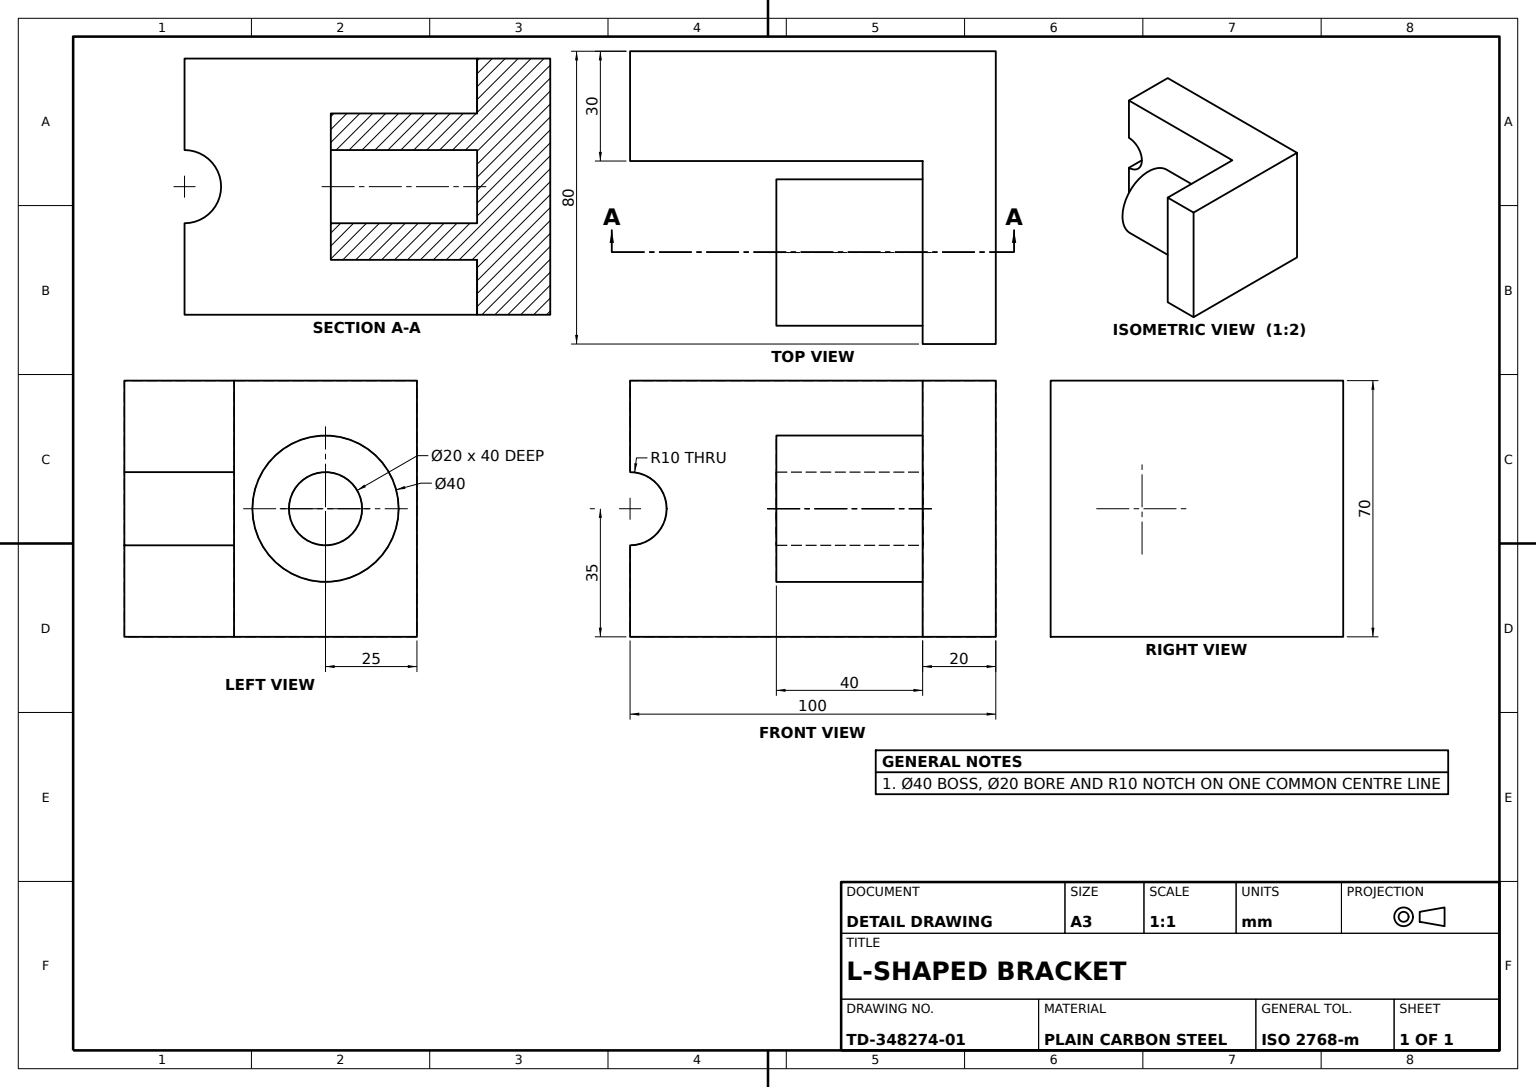
from build123d import *

# Parameters (mm, degrees)
BASE_PLATE_SKETCH_W        = 100
BASE_PLATE_SKETCH_H        = 70
BASE_PLATE_DEPTH           = 30
SEMICIRCULAR_NOTCH_DEPTH   = 30
UPRIGHT_WALL_SKETCH_W      = 50
UPRIGHT_WALL_SKETCH_H      = 70
UPRIGHT_WALL_DEPTH         = 20
HALF_ROUND_BOSS_SKETCH_R   = 20
HALF_ROUND_BOSS_SKETCH_R_2 = 10
HALF_ROUND_BOSS_DEPTH      = 40


with BuildPart() as part:
    # Base Plate Sketch → Base Plate (new body)
    with BuildSketch(Plane.XY):
        with Locations((50, 35)):
            Rectangle(BASE_PLATE_SKETCH_W, BASE_PLATE_SKETCH_H)
    extrude(amount=BASE_PLATE_DEPTH)

    # Notch Sketch → Semicircular Notch (cut)
    with BuildSketch(Plane.XY.offset(30)):
        with BuildLine():
            Line((0, 45), (0, 25))
            ThreePointArc((0, 25), (10, 35), (0, 45))
        make_face()
    extrude(amount=-SEMICIRCULAR_NOTCH_DEPTH, mode=Mode.SUBTRACT)

    # Upright Wall Sketch → Upright Wall (add)
    with BuildSketch(Plane(origin=(100, 0, 0), x_dir=(0, 0, -1), z_dir=(1, 0, 0))):
        with Locations((-55, 35)):
            Rectangle(UPRIGHT_WALL_SKETCH_W, UPRIGHT_WALL_SKETCH_H)
    extrude(amount=-UPRIGHT_WALL_DEPTH)

    # Half-Round Boss Sketch → Half-Round Boss (add)
    with BuildSketch(Plane.ZY.offset(-80)):
        with Locations(Location((55, 35, 0), (0, 0, 180))):
            Circle(HALF_ROUND_BOSS_SKETCH_R)
        with Locations((55, 35)):
            Circle(HALF_ROUND_BOSS_SKETCH_R_2, mode=Mode.SUBTRACT)
    extrude(amount=HALF_ROUND_BOSS_DEPTH)


solid = part.part
